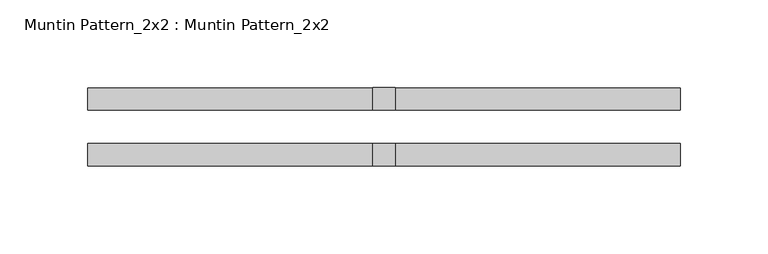
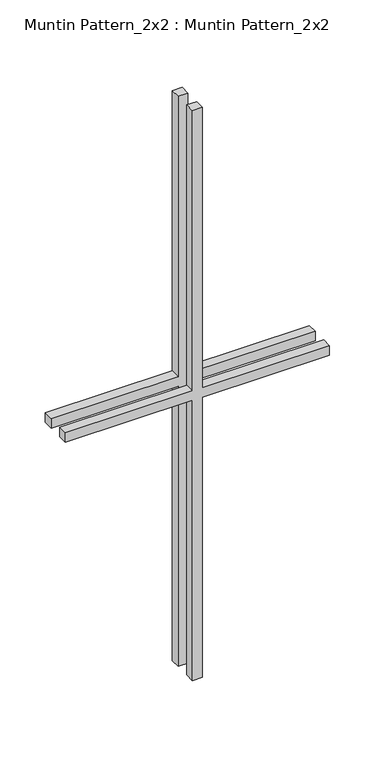
"""IFC4 building model written with IfcOpenShell, lengths in millimetres: proxy geometry, Muntin Pattern_2x2 : Muntin Pattern_2x2."""

from ifc_helpers import new_model, si_unit, frame, origin, place, context, project, spatial, polyline, outline, extrude, source, transform, mapped, element, save


def muntin_pattern_2x2_muntin_pattern_2x2_6186d23a(model_context):
    return source(origin(), model_context, "Body", "SweptSolid", [
        extrude(outline(polyline([(390.525, -6.35), (390.525, -168.275), (377.825, -168.275), (377.825, -6.35), (0.0, -6.35), (0.0, 6.35), (377.825, 6.35), (377.825, 168.275), (390.525, 168.275), (390.525, 6.35), (768.35, 6.35), (768.35, -6.35), (390.525, -6.35)])), frame((0.0, 9.525, 0.0), z_axis=(0.0, 1.0, 0.0), x_axis=(0.0, 0.0, 1.0)), (0.0, 0.0, 1.0), 12.7),
        extrude(outline(polyline([(390.525, -6.35), (390.525, -168.275), (377.825, -168.275), (377.825, -6.35), (0.0, -6.35), (0.0, 6.35), (377.825, 6.35), (377.825, 168.275), (390.525, 168.275), (390.525, 6.35), (768.35, 6.35), (768.35, -6.35), (390.525, -6.35)])), frame((0.0, -22.225, 0.0), z_axis=(0.0, 1.0, 0.0), x_axis=(0.0, 0.0, 1.0)), (0.0, 0.0, 1.0), 12.7),
    ])


if __name__ == "__main__":
    model = new_model("IFC4")
    model_context = context("Model", 3, world=origin())
    ifc_project = project(units=[si_unit("LENGTHUNIT", "METRE", prefix="MILLI")], contexts=[model_context])
    site = spatial("IfcSite", under=ifc_project)
    building = spatial("IfcBuilding", under=site)
    placement = place(None, origin())
    muntin_pattern_2x2_muntin_pattern_2x2_shape = muntin_pattern_2x2_muntin_pattern_2x2_6186d23a(model_context)
    element("IfcBuildingElementProxy", 1, Name="Muntin Pattern_2x2 : Muntin Pattern_2x2", ObjectType="Muntin Pattern_2x2 : Muntin Pattern_2x2", at=placement, inside=building, context=model_context, shape_type="MappedRepresentation", body=[
        mapped(muntin_pattern_2x2_muntin_pattern_2x2_shape, transform((0.0, 0.0, 0.0), x_axis=(1.0, 0.0, 0.0), y_axis=(0.0, 1.0, 0.0), z_axis=(0.0, 0.0, 1.0))),
    ])
    save(model, "model.ifc")

# Revit data of these elements
# Type "Muntin Pattern_2x2 : Muntin Pattern_2x2"
#   Width [instance default] = 4' - 0"
#   Thickness = 0' - 0 1/2"
#   Height [instance default] = 4' - 0"
#   Distance = 0' - 0 3/4"
#   Interior Material [instance default] = none
#   Exterior Material [instance default] = none
#   Default Elevation = 0
# Element 1 (IfcBuildingElementProxy, "Muntin Pattern_2x2 : Muntin Pattern_2x2")
#   Width = 1' - 1 1/4"
#   Height = 2' - 6 1/4"
#   Interior Material = Wood - Stained
#   Exterior Material = Clad - White
#   Materials on its faces: "Clad - White", "Wood - Stained"
# Materials
#   "Clad - White": class "Wood", colour RGB 242 242 238, transparency 0, Cost = 0
#   "Wood - Stained": class "Wood", colour RGB 224 178 126, transparency 0, Cost = 0
